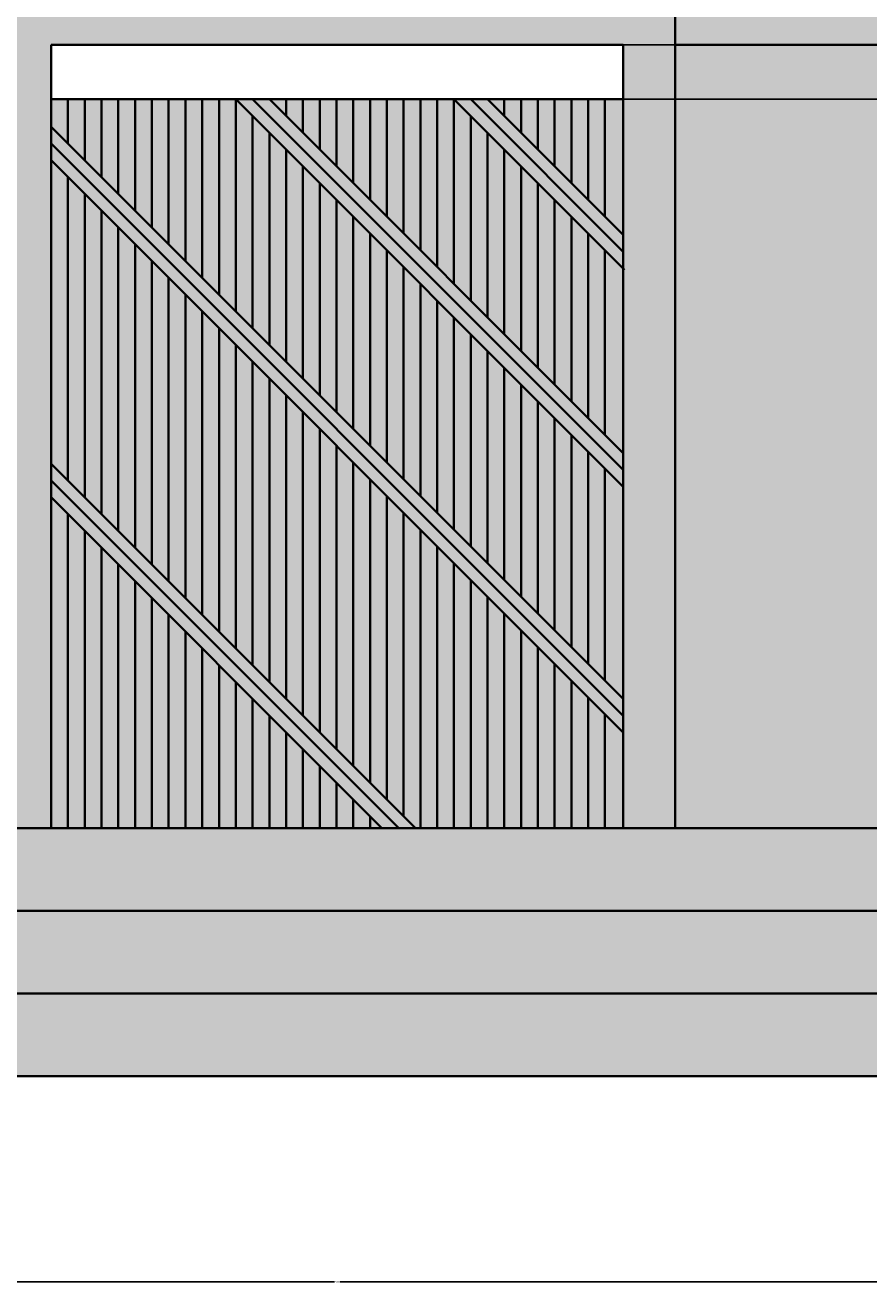
# Model space of a CAD drawing. Units: feet. Extents: x 2893 to 4112, y 897 to 1573.
# Tile 2 of 7: x 3123 to 3253, y 897 to 1090. Entities that reach past the tile are written whole.
import ezdxf

# ---------------------------------------------------------------- set-up
doc = ezdxf.new("R2010")
doc.units = ezdxf.units.FT
for name, color, linetype, lineweight in [('A-ANNO-DIMS', 2, 'Continuous', 18), ('A-ELEV', 7, 'Continuous', 35), ('A-ELEV-PATT', 8, 'Continuous', 13)]:
    doc.layers.add(name, color=color, linetype=linetype, lineweight=lineweight)
doc.styles.get("Standard").update_dxf_attribs({"font": 'arial.ttf'})
doc.dimstyles.get("Standard").update_dxf_attribs({"dimtxt": 0.18, "dimasz": 0.18, "dimexe": 0.18, "dimexo": 0.0625, "dimgap": 0.09, "dimtad": 0, "dimtih": 1, "dimtoh": 1, "dimdec": 1, "dimzin": 0, "dimdsep": 46, "dimlunit": 3, "dimtxsty": 'Standard', "dimcen": 0.09, "dimadec": 0, "dimazin": 0, "dimtfac": 1, "dimtdec": 1, "dimtofl": 0, "dimtmove": 0, "dimatfit": 3, "dimfxl": 1, "dimtolj": 1, "dimtzin": 0, "dimarcsym": 0})

# ---------------------------------------------------------------- blocks, each defined once
blk = doc.blocks.new('*D48')
at = {"layer": 'A-ANNO-DIMS', "color": 0, "lineweight": -2, "transparency": 16777216}
for p, q in [((2924.72, 1491.83), (2924.72, 897.37)), ((3417.56, 1491.83), (3417.56, 897.37)), ((2924.9, 897.55), (3170.74, 897.55)), ((3417.38, 897.55), (3171.54, 897.55))]:
    blk.add_line(p, q, dxfattribs=at)
at = {"layer": 'A-ANNO-DIMS', "color": 0, "transparency": 16777216}
for points in [[(2924.9, 897.58), (2924.9, 897.52), (2924.72, 897.55)], [(3417.38, 897.58), (3417.38, 897.52), (3417.56, 897.55)]]:
    blk.add_solid(points, dxfattribs=at)
at = {"layer": 'Defpoints', "color": 0, "transparency": 16777216}
for p in [(2924.72, 1491.89), (3417.56, 1491.89), (3417.56, 897.55)]:
    blk.add_point(p, dxfattribs=at)
at = {"layer": 'A-ANNO-DIMS', "color": 0, "transparency": 16777216, "insert": (3171.14, 897.55), "char_height": 0.18, "attachment_point": 5}
blk.add_mtext('\\A1;492.8', dxfattribs=at)
blk = doc.blocks.new('*D49')
at = {"layer": 'A-ANNO-DIMS', "color": 0, "lineweight": -2, "transparency": 16777216}
for p, q in [((3215.03, 1078.68), (3449.24, 1078.68)), ((3449.06, 1078.5), (3449.06, 1023.03)), ((3449.06, 967.19), (3449.06, 1022.66)), ((3215.03, 967.01), (3449.24, 967.01))]:
    blk.add_line(p, q, dxfattribs=at)
at = {"layer": 'A-ANNO-DIMS', "color": 0, "transparency": 16777216}
for points in [[(3449.03, 1078.5), (3449.09, 1078.5), (3449.06, 1078.68)], [(3449.03, 967.19), (3449.09, 967.19), (3449.06, 967.01)]]:
    blk.add_solid(points, dxfattribs=at)
at = {"layer": 'Defpoints', "color": 0, "transparency": 16777216}
for p in [(3214.97, 1078.68), (3449.06, 1078.68), (3214.97, 967.01)]:
    blk.add_point(p, dxfattribs=at)
at = {"layer": 'A-ANNO-DIMS', "color": 0, "transparency": 16777216, "insert": (3449.06, 1022.85), "char_height": 0.18, "attachment_point": 5}
blk.add_mtext('\\A1;111.66', dxfattribs=at)
blk = doc.blocks.new('*D50')
at = {"layer": 'A-ANNO-DIMS', "color": 0, "lineweight": -2, "transparency": 16777216}
for p, q in [((3215.03, 1087.01), (3449.24, 1087.01)), ((3449.06, 1086.83), (3449.06, 1083.03)), ((3449.06, 1078.86), (3449.06, 1082.66)), ((3215.03, 1078.68), (3449.24, 1078.68))]:
    blk.add_line(p, q, dxfattribs=at)
at = {"layer": 'A-ANNO-DIMS', "color": 0, "transparency": 16777216}
for points in [[(3449.03, 1086.83), (3449.09, 1086.83), (3449.06, 1087.01)], [(3449.03, 1078.86), (3449.09, 1078.86), (3449.06, 1078.68)]]:
    blk.add_solid(points, dxfattribs=at)
at = {"layer": 'Defpoints', "color": 0, "transparency": 16777216}
for p in [(3214.97, 1087.01), (3449.06, 1087.01), (3214.97, 1078.68)]:
    blk.add_point(p, dxfattribs=at)
at = {"layer": 'A-ANNO-DIMS', "color": 0, "transparency": 16777216, "insert": (3449.06, 1082.85), "char_height": 0.18, "attachment_point": 5}
blk.add_mtext('\\A1;8.338', dxfattribs=at)
blk = doc.blocks.new('*D51')
at = {"layer": 'A-ANNO-DIMS', "color": 0, "lineweight": -2, "transparency": 16777216}
for p, q in [((3189.38, 1112.11), (3449.24, 1112.11)), ((3449.06, 1111.93), (3449.06, 1099.74)), ((3449.06, 1087.19), (3449.06, 1099.38)), ((3215.03, 1087.01), (3449.24, 1087.01))]:
    blk.add_line(p, q, dxfattribs=at)
at = {"layer": 'A-ANNO-DIMS', "color": 0, "transparency": 16777216}
for points in [[(3449.03, 1111.93), (3449.09, 1111.93), (3449.06, 1112.11)], [(3449.03, 1087.19), (3449.09, 1087.19), (3449.06, 1087.01)]]:
    blk.add_solid(points, dxfattribs=at)
at = {"layer": 'Defpoints', "color": 0, "transparency": 16777216}
for p in [(3189.32, 1112.11), (3449.06, 1112.11), (3214.97, 1087.01)]:
    blk.add_point(p, dxfattribs=at)
at = {"layer": 'A-ANNO-DIMS', "color": 0, "transparency": 16777216, "insert": (3449.06, 1099.56), "char_height": 0.18, "attachment_point": 5}
blk.add_mtext('\\A1;25.095', dxfattribs=at)

msp = doc.modelspace()

# ---------------------------------------------------------------- hatches: boundary and pattern name
at = {"layer": 'A-ELEV-PATT'}
h = msp.add_hatch(color=256, dxfattribs=at)
h.dxf.hatch_style = 1
h.paths.add_polyline_path([(3222.9589, 1541.1646), (3119.3255, 1541.1646), (3119.3255, 967.0143), (3127.3151, 967.0143), (3127.3151, 1087.0143), (3214.9693, 1087.0143), (3214.9693, 1078.6766), (3214.9693, 967.0143), (3222.9589, 967.0143)])
h.paths.add_polyline_path([(3152.9675, 1482.3616), (3189.3169, 1482.3616), (3189.3169, 1457.0324), (3189.3169, 1377.2236), (3152.9675, 1377.2236), (3152.9675, 1457.0324)], flags=16)
h.paths.add_polyline_path([(3155.237, 1480.0922), (3187.0474, 1480.0922), (3187.0474, 1459.3019), (3155.237, 1459.3019)], flags=0)
h.paths.add_polyline_path([(3155.237, 1454.7629), (3187.0474, 1454.7629), (3187.0474, 1379.4931), (3155.237, 1379.4931)], flags=0)
h.paths.add_polyline_path([(3152.9675, 1354.8437), (3189.3169, 1354.8437), (3189.3169, 1329.5145), (3189.3169, 1249.7057), (3152.9675, 1249.7057), (3152.9675, 1329.5145)], flags=16)
h.paths.add_polyline_path([(3155.237, 1352.5742), (3187.0474, 1352.5742), (3187.0474, 1331.784), (3155.237, 1331.784)], flags=0)
h.paths.add_polyline_path([(3155.237, 1327.245), (3187.0474, 1327.245), (3187.0474, 1251.9752), (3155.237, 1251.9752)], flags=0)
h.paths.add_polyline_path([(3152.9675, 1217.2478), (3189.3169, 1217.2478), (3189.3169, 1191.9186), (3189.3169, 1112.1098), (3152.9675, 1112.1098), (3152.9675, 1191.9186)], flags=16)
h.paths.add_polyline_path([(3155.237, 1214.9783), (3187.0474, 1214.9783), (3187.0474, 1194.1881), (3155.237, 1194.1881)], flags=0)
h.paths.add_polyline_path([(3155.237, 1189.6491), (3187.0474, 1189.6491), (3187.0474, 1114.3793), (3155.237, 1114.3793)], flags=0)
h = msp.add_hatch(dxfattribs=at)
h.set_pattern_fill('AR-BRELM', color=256, scale=0.1)
h.set_pattern_definition([(0, (-663.002, 0), (0, 13.5484), [19.3675, -0.9525]), (0, (-663.002, 5.715), (0, 13.5484), [19.3675, -0.9525]), (0, (-657.922, 6.774), (0, 13.5484), [9.2075, -0.9525]), (0, (-657.922, 12.489), (0, 13.5484), [9.2075, -0.9525]), (90, (-663.002, 0), (-20.32, 1e-15), [5.715, -7.8334]), (90, (-663.954, 0), (-20.32, 1e-15), [5.715, -7.8334]), (90, (-657.922, 6.774), (-10.16, 6e-16), [5.715, -7.8334]), (90, (-658.874, 6.774), (-10.16, 6e-16), [5.715, -7.8334])])
h.paths.add_polyline_path([(3222.9589, 1541.1646), (3119.3255, 1541.1646), (3119.3255, 967.0143), (3127.3151, 967.0143), (3127.3151, 1087.0143), (3214.9693, 1087.0143), (3214.9693, 1078.6766), (3214.9693, 967.0143), (3222.9589, 967.0143)])
h.paths.add_polyline_path([(3152.9675, 1482.3616), (3189.3169, 1482.3616), (3189.3169, 1457.0324), (3189.3169, 1377.2236), (3152.9675, 1377.2236), (3152.9675, 1457.0324)], flags=16)
h.paths.add_polyline_path([(3155.237, 1480.0922), (3187.0474, 1480.0922), (3187.0474, 1459.3019), (3155.237, 1459.3019)], flags=0)
h.paths.add_polyline_path([(3155.237, 1454.7629), (3187.0474, 1454.7629), (3187.0474, 1379.4931), (3155.237, 1379.4931)], flags=0)
h.paths.add_polyline_path([(3152.9675, 1354.8437), (3189.3169, 1354.8437), (3189.3169, 1329.5145), (3189.3169, 1249.7057), (3152.9675, 1249.7057), (3152.9675, 1329.5145)], flags=16)
h.paths.add_polyline_path([(3155.237, 1352.5742), (3187.0474, 1352.5742), (3187.0474, 1331.784), (3155.237, 1331.784)], flags=0)
h.paths.add_polyline_path([(3155.237, 1327.245), (3187.0474, 1327.245), (3187.0474, 1251.9752), (3155.237, 1251.9752)], flags=0)
h.paths.add_polyline_path([(3152.9675, 1217.2478), (3189.3169, 1217.2478), (3189.3169, 1191.9186), (3189.3169, 1112.1098), (3152.9675, 1112.1098), (3152.9675, 1191.9186)], flags=16)
h.paths.add_polyline_path([(3155.237, 1214.9783), (3187.0474, 1214.9783), (3187.0474, 1194.1881), (3155.237, 1194.1881)], flags=0)
h.paths.add_polyline_path([(3155.237, 1189.6491), (3187.0474, 1189.6491), (3187.0474, 1114.3793), (3155.237, 1114.3793)], flags=0)
h = msp.add_hatch(color=256, dxfattribs=at)
h.dxf.hatch_style = 1
h.paths.add_polyline_path([(3119.3255, 1527.889), (2924.7207, 1527.889), (2924.7207, 1491.889), (3119.3255, 1491.889)])
h.paths.add_polyline_path([(3417.5637, 1527.889), (3222.9589, 1527.889), (3222.9589, 1491.889), (3417.5637, 1491.889)])
h.paths.add_polyline_path([(3119.3255, 1102.9302), (2946.0771, 1102.9302), (2946.0771, 1139.3799), (2934.0287, 1139.3799), (2934.0287, 1093.0143), (3119.3255, 1093.0143)])
h.paths.add_polyline_path([(3119.3255, 1093.0143), (2934.4679, 1093.0143), (2934.4679, 1087.0143), (3119.3255, 1087.0143)])
h.paths.add_polyline_path([(3408.2557, 1139.3799), (3396.2073, 1139.3799), (3396.2073, 1136.9984), (3396.2073, 1102.9302), (3222.9589, 1102.9302), (3222.9589, 1093.0143), (3408.2557, 1093.0143)])
h.paths.add_polyline_path([(3407.8165, 1093.0143), (3222.9589, 1093.0143), (3222.9589, 1087.0143), (3407.8165, 1087.0143)])
h = msp.add_hatch(color=256, dxfattribs=at)
h.dxf.hatch_style = 1
h.paths.add_polyline_path([(3390.4511, 1087.0143), (3222.9589, 1087.0143), (3222.9589, 967.0143), (3255.8959, 967.0143), (3255.8959, 1053.0375), (3262.7641, 1053.0375), (3364.4735, 1053.0375), (3364.4735, 967.0143), (3390.4511, 967.0143)])
h.paths.add_polyline_path([(3119.3255, 1087.0143), (2951.8333, 1087.0143), (2951.8333, 967.0143), (2977.8109, 967.0143), (2977.8109, 1053.0375), (2984.6791, 1053.0375), (3086.3885, 1053.0375), (3086.3885, 967.0143), (3119.3255, 967.0143)])
h = msp.add_hatch(color=256, dxfattribs=at)
h.dxf.hatch_style = 1
h.paths.add_polyline_path([(3189.0392, 1078.6766), (3186.4674, 1078.6766), (3186.4674, 1052.9582), (3189.0392, 1050.3864)], flags=16)
h.paths.add_polyline_path([(3186.4674, 1078.6766), (3183.8955, 1078.6766), (3183.8955, 1055.5301), (3186.4674, 1052.9582)], flags=16)
h.paths.add_polyline_path([(3183.8955, 1078.6766), (3181.3237, 1078.6766), (3181.3237, 1058.1019), (3183.8955, 1055.5301)], flags=16)
h.paths.add_polyline_path([(3181.3237, 1078.6766), (3178.7518, 1078.6766), (3178.7518, 1060.6737), (3181.3237, 1058.1019)], flags=16)
h.paths.add_polyline_path([(3178.7518, 1078.6766), (3176.18, 1078.6766), (3176.18, 1063.2456), (3178.7518, 1060.6737)], flags=16)
h.paths.add_polyline_path([(3176.18, 1078.6766), (3173.6082, 1078.6766), (3173.6082, 1065.8174), (3176.18, 1063.2456)], flags=16)
h.paths.add_polyline_path([(3173.6082, 1078.6766), (3171.0363, 1078.6766), (3171.0363, 1068.3892), (3173.6082, 1065.8174)], flags=16)
h.paths.add_polyline_path([(3171.0363, 1078.6766), (3168.4645, 1078.6766), (3168.4645, 1070.9611), (3171.0363, 1068.3892)], flags=16)
h.paths.add_polyline_path([(3168.4645, 1078.6766), (3165.8926, 1078.6766), (3165.8926, 1073.5329), (3168.4645, 1070.9611)], flags=16)
h.paths.add_polyline_path([(3165.8926, 1078.6766), (3163.3208, 1078.6766), (3163.3208, 1076.1048), (3165.8926, 1073.5329)], flags=16)
h.paths.add_polyline_path([(3163.3208, 1078.6766), (3160.749, 1078.6766), (3163.3208, 1076.1048)], flags=16)
h.paths.add_polyline_path([(3160.749, 1078.6766), (3158.1771, 1078.6766), (3214.9693, 1021.8844), (3214.9693, 1024.4562)], flags=17)
h.paths.add_polyline_path([(3158.1771, 1078.6766), (3155.6053, 1078.6766), (3214.9693, 1019.3125), (3214.9693, 1021.8844)])
h.paths.add_polyline_path([(3196.7547, 1037.5272), (3194.1829, 1040.099), (3194.1829, 1007.596), (3196.7547, 1005.0242)], flags=17)
h.paths.add_polyline_path([(3199.3266, 1034.9553), (3196.7547, 1037.5272), (3196.7547, 1005.0242), (3199.3266, 1002.4523)], flags=17)
h.paths.add_polyline_path([(3201.8984, 1032.3835), (3199.3266, 1034.9553), (3199.3266, 1002.4523), (3201.8984, 999.8805)], flags=17)
h.paths.add_polyline_path([(3204.4702, 1029.8117), (3201.8984, 1032.3835), (3201.8984, 999.8805), (3204.4702, 997.3086)], flags=17)
h.paths.add_polyline_path([(3207.0421, 1027.2398), (3204.4702, 1029.8117), (3204.4702, 997.3086), (3207.0421, 994.7368)], flags=17)
h.paths.add_polyline_path([(3209.6139, 1024.668), (3207.0421, 1027.2398), (3207.0421, 994.7368), (3209.6139, 992.165)], flags=17)
h.paths.add_polyline_path([(3212.1857, 1022.0961), (3209.6139, 1024.668), (3209.6139, 992.165), (3212.1857, 989.5931)], flags=17)
h.paths.add_polyline_path([(3214.9693, 1019.3125), (3212.1857, 1022.0961), (3212.1857, 989.5931), (3214.9693, 986.8095)], flags=17)
h.paths.add_polyline_path([(3173.6082, 1060.6737), (3171.0363, 1063.2456), (3171.0363, 1030.7426), (3173.6082, 1028.1707)], flags=17)
h.paths.add_polyline_path([(3176.18, 1058.1019), (3173.6082, 1060.6737), (3173.6082, 1028.1707), (3176.18, 1025.5989)], flags=17)
h.paths.add_polyline_path([(3178.7518, 1055.5301), (3176.18, 1058.1019), (3176.18, 1025.5989), (3178.7518, 1023.027)], flags=17)
h.paths.add_polyline_path([(3181.3237, 1052.9582), (3178.7518, 1055.5301), (3178.7518, 1023.027), (3181.3237, 1020.4552)], flags=17)
h.paths.add_polyline_path([(3183.8955, 1050.3864), (3181.3237, 1052.9582), (3181.3237, 1020.4552), (3183.8955, 1017.8834)], flags=17)
h.paths.add_polyline_path([(3186.4674, 1047.8145), (3183.8955, 1050.3864), (3183.8955, 1017.8834), (3186.4674, 1015.3115)], flags=17)
h.paths.add_polyline_path([(3189.0392, 1045.2427), (3186.4674, 1047.8145), (3186.4674, 1015.3115), (3189.0392, 1012.7397)], flags=17)
h.paths.add_polyline_path([(3191.611, 1042.6709), (3189.0392, 1045.2427), (3189.0392, 1012.7397), (3191.611, 1010.1678)], flags=17)
h.paths.add_polyline_path([(3194.1829, 1040.099), (3191.611, 1042.6709), (3191.611, 1010.1678), (3194.1829, 1007.596)], flags=17)
h.paths.add_polyline_path([(3171.0363, 1063.2456), (3168.4645, 1065.8174), (3168.4645, 1033.3144), (3171.0363, 1030.7426)], flags=17)
h.paths.add_polyline_path([(3168.4645, 1065.8174), (3165.8926, 1068.3892), (3165.8926, 1035.8862), (3168.4645, 1033.3144)], flags=17)
h.paths.add_polyline_path([(3165.8926, 1068.3892), (3163.3208, 1070.9611), (3163.3208, 1038.4581), (3165.8926, 1035.8862)], flags=17)
h.paths.add_polyline_path([(3163.3208, 1070.9611), (3160.749, 1073.5329), (3160.749, 1041.0299), (3163.3208, 1038.4581)], flags=17)
h.paths.add_polyline_path([(3160.749, 1073.5329), (3158.1771, 1076.1048), (3158.1771, 1043.6018), (3160.749, 1041.0299)], flags=16)
h.paths.add_polyline_path([(3158.1771, 1076.1048), (3155.6053, 1078.6766), (3155.6053, 1046.1736), (3158.1771, 1043.6018)], flags=17)
h.paths.add_polyline_path([(3155.6053, 1078.6766), (3153.0334, 1078.6766), (3153.0334, 1048.7454), (3155.6053, 1046.1736)])
h.paths.add_polyline_path([(3153.0334, 1078.6766), (3150.4616, 1078.6766), (3150.4616, 1051.3173), (3153.0334, 1048.7454)])
h.paths.add_polyline_path([(3150.4616, 1078.6766), (3147.8898, 1078.6766), (3147.8898, 1053.8891), (3150.4616, 1051.3173)])
h.paths.add_polyline_path([(3147.8898, 1078.6766), (3145.3179, 1078.6766), (3145.3179, 1056.4609), (3147.8898, 1053.8891)])
h.paths.add_polyline_path([(3145.3179, 1078.6766), (3142.7461, 1078.6766), (3142.7461, 1059.0328), (3145.3179, 1056.4609)])
h.paths.add_polyline_path([(3140.1742, 1078.6766), (3137.6024, 1078.6766), (3137.6024, 1064.1765), (3140.1742, 1061.6046)])
h.paths.add_polyline_path([(3142.7461, 1078.6766), (3140.1742, 1078.6766), (3140.1742, 1061.6046), (3142.7461, 1059.0328)])
h.paths.add_polyline_path([(3137.6024, 1078.6766), (3135.0306, 1078.6766), (3135.0306, 1066.7483), (3137.6024, 1064.1765)])
h.paths.add_polyline_path([(3135.0306, 1078.6766), (3132.4587, 1078.6766), (3132.4587, 1069.3201), (3135.0306, 1066.7483)])
h.paths.add_polyline_path([(3129.8869, 1078.6766), (3127.3151, 1078.6766), (3127.3151, 1074.4638), (3129.8869, 1071.892)])
h.paths.add_polyline_path([(3132.4587, 1078.6766), (3129.8869, 1078.6766), (3129.8869, 1071.892), (3132.4587, 1069.3201)])
h.paths.add_polyline_path([(3127.3151, 1074.4638), (3127.3151, 1071.892), (3214.9693, 984.2377), (3214.9693, 986.8095)])
h.paths.add_polyline_path([(3176.18, 968.8368), (3176.18, 967.0143), (3178.0025, 967.0143)], flags=16)
h.paths.add_polyline_path([(3176.18, 968.8368), (3173.6082, 971.4087), (3173.6082, 967.0143), (3176.18, 967.0143)], flags=16)
h.paths.add_polyline_path([(3173.6082, 971.4087), (3171.0363, 973.9805), (3171.0363, 967.0143), (3173.6082, 967.0143)], flags=16)
h.paths.add_polyline_path([(3171.0363, 973.9805), (3168.4645, 976.5524), (3168.4645, 967.0143), (3171.0363, 967.0143)], flags=16)
h.paths.add_polyline_path([(3168.4645, 976.5524), (3165.8926, 979.1242), (3165.8926, 967.0143), (3168.4645, 967.0143)], flags=16)
h.paths.add_polyline_path([(3165.8926, 979.1242), (3163.3208, 981.696), (3163.3208, 967.0143), (3165.8926, 967.0143)], flags=16)
h.paths.add_polyline_path([(3163.3208, 981.696), (3160.749, 984.2679), (3160.749, 967.0143), (3163.3208, 967.0143)], flags=16)
h.paths.add_polyline_path([(3160.749, 984.2679), (3158.1771, 986.8397), (3158.1771, 967.0143), (3160.749, 967.0143)], flags=16)
h.paths.add_polyline_path([(3158.1771, 986.8397), (3155.6053, 989.4116), (3155.6053, 967.0143), (3158.1771, 967.0143)], flags=16)
h.paths.add_polyline_path([(3155.6053, 989.4116), (3153.0334, 991.9834), (3153.0334, 967.0143), (3155.6053, 967.0143)], flags=16)
h.paths.add_polyline_path([(3153.0334, 991.9834), (3150.4616, 994.5552), (3150.4616, 967.0143), (3153.0334, 967.0143)], flags=16)
h.paths.add_polyline_path([(3127.3151, 1020.2736), (3127.3151, 1017.7018), (3178.0025, 967.0143), (3180.5744, 967.0143)], flags=17)
h.paths.add_polyline_path([(3127.3151, 1022.8455), (3127.3151, 1020.2736), (3180.5744, 967.0143), (3183.1462, 967.0143)])
h = msp.add_hatch(color=256, dxfattribs=at)
h.dxf.hatch_style = 1
h.paths.add_polyline_path([(3214.9693, 1078.6766), (3212.1857, 1078.6766), (3212.1857, 1060.6737), (3214.9693, 1057.8901)], flags=16)
h.paths.add_polyline_path([(3212.1857, 1078.6766), (3209.6139, 1078.6766), (3209.6139, 1063.2456), (3212.1857, 1060.6737)], flags=16)
h.paths.add_polyline_path([(3209.6139, 1078.6766), (3207.0421, 1078.6766), (3207.0421, 1065.8174), (3209.6139, 1063.2456)], flags=16)
h.paths.add_polyline_path([(3207.0421, 1078.6766), (3204.4702, 1078.6766), (3204.4702, 1068.3892), (3207.0421, 1065.8174)], flags=16)
h.paths.add_polyline_path([(3204.4702, 1078.6766), (3201.8984, 1078.6766), (3201.8984, 1070.9611), (3204.4702, 1068.3892)], flags=16)
h.paths.add_polyline_path([(3201.8984, 1078.6766), (3199.3266, 1078.6766), (3199.3266, 1073.5329), (3201.8984, 1070.9611)], flags=16)
h.paths.add_polyline_path([(3199.3266, 1078.6766), (3196.7547, 1078.6766), (3196.7547, 1076.1048), (3199.3266, 1073.5329)], flags=16)
h.paths.add_polyline_path([(3196.7547, 1078.6766), (3194.1829, 1078.6766), (3196.7547, 1076.1048)], flags=16)
h.paths.add_polyline_path([(3196.7547, 1076.1048), (3194.1829, 1078.6766), (3191.611, 1078.6766), (3214.9693, 1055.3183), (3214.9693, 1057.8901), (3212.1857, 1060.6737), (3209.6139, 1063.2456), (3207.0421, 1065.8174), (3204.4702, 1068.3892), (3201.8984, 1070.9611), (3199.3266, 1073.5329)], flags=17)
h.paths.add_polyline_path([(3191.611, 1078.6766), (3189.0392, 1078.6766), (3214.9693, 1052.7465), (3214.9693, 1055.3183)])
h.paths.add_polyline_path([(3214.9693, 1052.7465), (3212.1857, 1055.5301), (3212.1857, 1027.2398), (3214.9693, 1024.4562)])
h.paths.add_polyline_path([(3212.1857, 1055.5301), (3209.6139, 1058.1019), (3209.6139, 1029.8117), (3212.1857, 1027.2398)])
h.paths.add_polyline_path([(3209.6139, 1058.1019), (3207.0421, 1060.6737), (3207.0421, 1032.3835), (3209.6139, 1029.8117)])
h.paths.add_polyline_path([(3207.0421, 1060.6737), (3204.4702, 1063.2456), (3204.4702, 1034.9553), (3207.0421, 1032.3835)])
h.paths.add_polyline_path([(3204.4702, 1063.2456), (3201.8984, 1065.8174), (3201.8984, 1037.5272), (3204.4702, 1034.9553)])
h.paths.add_polyline_path([(3201.8984, 1065.8174), (3199.3266, 1068.3892), (3199.3266, 1040.099), (3201.8984, 1037.5272)])
h.paths.add_polyline_path([(3199.3266, 1068.3892), (3196.7547, 1070.9611), (3196.7547, 1042.6709), (3199.3266, 1040.099)])
h.paths.add_polyline_path([(3196.7547, 1070.9611), (3194.1829, 1073.5329), (3194.1829, 1045.2427), (3196.7547, 1042.6709)])
h.paths.add_polyline_path([(3194.1829, 1073.5329), (3191.611, 1076.1048), (3191.611, 1047.8145), (3194.1829, 1045.2427)])
h.paths.add_polyline_path([(3191.611, 1076.1048), (3189.0392, 1078.6766), (3189.0392, 1050.3864), (3191.611, 1047.8145)])
h = msp.add_hatch(color=256, dxfattribs=at)
h.dxf.hatch_style = 1
h.paths.add_polyline_path([(3129.8869, 1015.13), (3127.3151, 1017.7018), (3127.3151, 967.0143), (3129.8869, 967.0143)])
h.paths.add_polyline_path([(3132.4587, 1012.5581), (3129.8869, 1015.13), (3129.8869, 967.0143), (3132.4587, 967.0143)])
h.paths.add_polyline_path([(3135.0306, 1009.9863), (3132.4587, 1012.5581), (3132.4587, 967.0143), (3135.0306, 967.0143)])
h.paths.add_polyline_path([(3137.6024, 1007.4144), (3135.0306, 1009.9863), (3135.0306, 967.0143), (3137.6024, 967.0143)])
h.paths.add_polyline_path([(3173.6082, 1023.027), (3171.0363, 1025.5989), (3171.0363, 979.1242), (3173.6082, 976.5524)])
h.paths.add_polyline_path([(3171.0363, 1025.5989), (3168.4645, 1028.1707), (3168.4645, 981.696), (3171.0363, 979.1242)])
h.paths.add_polyline_path([(3168.4645, 1028.1707), (3165.8926, 1030.7426), (3165.8926, 984.2679), (3168.4645, 981.696)], flags=17)
h.paths.add_polyline_path([(3165.8926, 1030.7426), (3163.3208, 1033.3144), (3163.3208, 986.8397), (3165.8926, 984.2679)], flags=17)
h.paths.add_polyline_path([(3163.3208, 1033.3144), (3160.749, 1035.8862), (3160.749, 989.4116), (3163.3208, 986.8397)], flags=17)
h.paths.add_polyline_path([(3160.749, 1035.8862), (3158.1771, 1038.4581), (3158.1771, 991.9834), (3160.749, 989.4116)], flags=17)
h.paths.add_polyline_path([(3158.1771, 1038.4581), (3155.6053, 1041.0299), (3155.6053, 994.5552), (3158.1771, 991.9834)], flags=17)
h.paths.add_polyline_path([(3155.6053, 1041.0299), (3153.0334, 1043.6018), (3153.0334, 997.1271), (3155.6053, 994.5552)], flags=17)
h.paths.add_polyline_path([(3153.0334, 1043.6018), (3150.4616, 1046.1736), (3150.4616, 999.6989), (3153.0334, 997.1271)], flags=17)
h.paths.add_polyline_path([(3150.4616, 1046.1736), (3147.8898, 1048.7454), (3147.8898, 1002.2708), (3150.4616, 999.6989)], flags=17)
h.paths.add_polyline_path([(3147.8898, 1048.7454), (3145.3179, 1051.3173), (3145.3179, 1004.8426), (3147.8898, 1002.2708)], flags=17)
h.paths.add_polyline_path([(3145.3179, 1051.3173), (3142.7461, 1053.8891), (3142.7461, 1007.4144), (3145.3179, 1004.8426)], flags=17)
h.paths.add_polyline_path([(3142.7461, 1053.8891), (3140.1742, 1056.4609), (3140.1742, 1009.9863), (3142.7461, 1007.4144)], flags=17)
h.paths.add_polyline_path([(3140.1742, 1056.4609), (3137.6024, 1059.0328), (3137.6024, 1012.5581), (3140.1742, 1009.9863)], flags=17)
h.paths.add_polyline_path([(3137.6024, 1059.0328), (3135.0306, 1061.6046), (3135.0306, 1015.13), (3137.6024, 1012.5581)], flags=17)
h.paths.add_polyline_path([(3127.3151, 1071.892), (3127.3151, 1069.3201), (3214.9693, 981.6659), (3214.9693, 984.2377)])
h = msp.add_hatch(color=256, dxfattribs=at)
h.dxf.hatch_style = 1
h.paths.add_polyline_path([(3132.4587, 1064.1765), (3129.8869, 1066.7483), (3129.8869, 1020.2736), (3132.4587, 1017.7018)])
h.paths.add_polyline_path([(3135.0306, 1061.6046), (3132.4587, 1064.1765), (3132.4587, 1017.7018), (3135.0306, 1015.13)])
h.paths.add_polyline_path([(3129.8869, 1066.7483), (3127.3151, 1069.3201), (3127.3151, 1022.8455), (3129.8869, 1020.2736)])
h = msp.add_hatch(color=256, dxfattribs=at)
h.dxf.hatch_style = 1
h.paths.add_polyline_path([(3214.9693, 981.6659), (3212.1857, 984.4494), (3212.1857, 967.0143), (3214.9693, 967.0143)])
h.paths.add_polyline_path([(3212.1857, 984.4494), (3209.6139, 987.0213), (3209.6139, 967.0143), (3212.1857, 967.0143)])
h.paths.add_polyline_path([(3209.6139, 987.0213), (3207.0421, 989.5931), (3207.0421, 967.0143), (3209.6139, 967.0143)])
h.paths.add_polyline_path([(3207.0421, 989.5931), (3204.4702, 992.165), (3204.4702, 967.0143), (3207.0421, 967.0143)])
h.paths.add_polyline_path([(3204.4702, 992.165), (3201.8984, 994.7368), (3201.8984, 967.0143), (3204.4702, 967.0143)])
h.paths.add_polyline_path([(3201.8984, 994.7368), (3199.3266, 997.3086), (3199.3266, 967.0143), (3201.8984, 967.0143)])
h.paths.add_polyline_path([(3199.3266, 997.3086), (3196.7547, 999.8805), (3196.7547, 967.0143), (3199.3266, 967.0143)])
h.paths.add_polyline_path([(3196.7547, 999.8805), (3194.1829, 1002.4523), (3194.1829, 967.0143), (3196.7547, 967.0143)])
h.paths.add_polyline_path([(3194.1829, 1002.4523), (3191.611, 1005.0242), (3191.611, 967.0143), (3194.1829, 967.0143)])
h.paths.add_polyline_path([(3191.611, 1005.0242), (3189.0392, 1007.596), (3189.0392, 967.0143), (3191.611, 967.0143)])
h.paths.add_polyline_path([(3189.0392, 1007.596), (3186.4674, 1010.1678), (3186.4674, 967.0143), (3189.0392, 967.0143)])
h.paths.add_polyline_path([(3186.4674, 1010.1678), (3183.8955, 1012.7397), (3183.8955, 967.0143), (3186.4674, 967.0143)])
h.paths.add_polyline_path([(3183.8955, 1012.7397), (3181.3237, 1015.3115), (3181.3237, 968.8368), (3183.1462, 967.0143), (3183.8955, 967.0143)])
h.paths.add_polyline_path([(3181.3237, 1015.3115), (3178.7518, 1017.8834), (3178.7518, 971.4087), (3181.3237, 968.8368)])
h.paths.add_polyline_path([(3178.7518, 1017.8834), (3176.18, 1020.4552), (3176.18, 973.9805), (3178.7518, 971.4087)])
h.paths.add_polyline_path([(3176.18, 1020.4552), (3173.6082, 1023.027), (3173.6082, 976.5524), (3176.18, 973.9805)])
h.paths.add_polyline_path([(3147.8898, 997.1271), (3145.3179, 999.6989), (3145.3179, 967.0143), (3147.8898, 967.0143)])
h.paths.add_polyline_path([(3150.4616, 994.5552), (3147.8898, 997.1271), (3147.8898, 967.0143), (3150.4616, 967.0143)])
h.paths.add_polyline_path([(3145.3179, 999.6989), (3142.7461, 1002.2708), (3142.7461, 967.0143), (3145.3179, 967.0143)])
h.paths.add_polyline_path([(3142.7461, 1002.2708), (3140.1742, 1004.8426), (3140.1742, 967.0143), (3142.7461, 967.0143)])
h.paths.add_polyline_path([(3140.1742, 1004.8426), (3137.6024, 1007.4144), (3137.6024, 967.0143), (3140.1742, 967.0143)])
h = msp.add_hatch(color=256, dxfattribs=at)
h.dxf.hatch_style = 1
h.paths.add_polyline_path([(3390.4511, 967.0143), (3222.9589, 967.0143), (2951.8333, 967.0143), (2932.7702, 954.3595), (3409.5142, 954.3595)])
h.paths.add_polyline_path([(3409.5142, 954.3595), (2932.7702, 954.3595), (2932.7702, 945.8624), (2926.5072, 941.7047), (3415.7772, 941.7047), (3409.5142, 945.8624)])
h.paths.add_polyline_path([(3415.7772, 941.7047), (2926.5072, 941.7047), (2926.5072, 929.0499), (3415.7772, 929.0499)])

# ---------------------------------------------------------------- linework, layer by layer
at = {"layer": 'A-ELEV'}
for p, q in [((3222.9589, 967.0143), (3222.9589, 1541.1646)), ((3214.9693, 1087.0143), (3127.3151, 1087.0143)), ((3214.9693, 1087.0143), (3127.3151, 1087.0143)), ((3214.9693, 1087.0143), (3127.3151, 1087.0143)), ((3407.8165, 1087.0143), (3222.9589, 1087.0143)), ((3129.8869, 1078.6766), (3129.8869, 1071.892)), ((3132.4587, 1078.6766), (3132.4587, 1069.3201)), ((3135.0306, 1078.6766), (3135.0306, 1066.7483)), ((3137.6024, 1078.6766), (3137.6024, 1064.1765)), ((3140.1742, 1078.6766), (3140.1742, 1061.6046)), ((3142.7461, 1078.6766), (3142.7461, 1059.0328)), ((3145.3179, 1078.6766), (3145.3179, 1056.4609)), ((3147.8898, 1078.6766), (3147.8898, 1053.8891)), ((3150.4616, 1078.6766), (3150.4616, 1051.3173)), ((3153.0334, 1078.6766), (3153.0334, 1048.7454)), ((3158.1771, 1078.6766), (3214.9693, 1021.8844)), ((3160.749, 1078.6766), (3214.9693, 1024.4562)), ((3163.3208, 1078.6766), (3163.3208, 1076.1048)), ((3163.3208, 1078.6766), (3163.3208, 1076.1048)), ((3165.8926, 1078.6766), (3165.8926, 1073.5329)), ((3168.4645, 1078.6766), (3168.4645, 1070.9611)), ((3171.0363, 1078.6766), (3171.0363, 1068.3892)), ((3173.6082, 1078.6766), (3173.6082, 1065.8174)), ((3176.18, 1078.6766), (3176.18, 1063.2456)), ((3178.7518, 1078.6766), (3178.7518, 1060.6737)), ((3181.3237, 1078.6766), (3181.3237, 1058.1019)), ((3183.8955, 1078.6766), (3183.8955, 1055.5301)), ((3186.4674, 1078.6766), (3186.4674, 1052.9582)), ((3191.611, 1078.6766), (3214.9693, 1055.3183)), ((3194.1829, 1078.6766), (3214.9693, 1057.8901)), ((3196.7547, 1078.6766), (3196.7547, 1076.1048)), ((3196.7547, 1078.6766), (3196.7547, 1076.1048)), ((3199.3266, 1078.6766), (3199.3266, 1073.5329)), ((3201.8984, 1078.6766), (3201.8984, 1070.9611)), ((3204.4702, 1078.6766), (3204.4702, 1068.3892)), ((3207.0421, 1078.6766), (3207.0421, 1065.8174)), ((3209.6139, 1078.6766), (3209.6139, 1063.2456)), ((3212.1857, 1078.6766), (3212.1857, 1060.6737)), ((3158.1771, 1076.1048), (3158.1771, 1043.6018)), ((3191.611, 1076.1048), (3191.611, 1047.8145)), ((3127.3151, 1074.4638), (3214.9693, 986.8095)), ((3160.749, 1073.5329), (3160.749, 1041.0299)), ((3194.1829, 1073.5329), (3194.1829, 1045.2427)), ((3127.3151, 1071.892), (3214.9693, 984.2377)), ((3127.3151, 1069.3201), (3214.9693, 981.6659)), ((3163.3208, 1070.9611), (3163.3208, 1038.4581)), ((3196.7547, 1070.9611), (3196.7547, 1042.6709)), ((3165.8926, 1068.3892), (3165.8926, 1035.8862)), ((3199.3266, 1068.3892), (3199.3266, 1040.099)), ((3129.8869, 1066.7483), (3129.8869, 1020.2736)), ((3168.4645, 1065.8174), (3168.4645, 1033.3144)), ((3201.8984, 1065.8174), (3201.8984, 1037.5272)), ((3132.4587, 1064.1765), (3132.4587, 1017.7018)), ((3135.0306, 1061.6046), (3135.0306, 1015.13)), ((3171.0363, 1063.2456), (3171.0363, 1030.7426)), ((3204.4702, 1063.2456), (3204.4702, 1034.9553)), ((3173.6082, 1060.6737), (3173.6082, 1028.1707)), ((3207.0421, 1060.6737), (3207.0421, 1032.3835)), ((3137.6024, 1059.0328), (3137.6024, 1012.5581)), ((3176.18, 1058.1019), (3176.18, 1025.5989)), ((3209.6139, 1058.1019), (3209.6139, 1029.8117)), ((3140.1742, 1056.4609), (3140.1742, 1009.9863)), ((3142.7461, 1053.8891), (3142.7461, 1007.4144)), ((3178.7518, 1055.5301), (3178.7518, 1023.027)), ((3212.1857, 1055.5301), (3212.1857, 1027.2398)), ((3181.3237, 1052.9582), (3181.3237, 1020.4552)), ((3145.3179, 1051.3173), (3145.3179, 1004.8426)), ((3183.8955, 1050.3864), (3183.8955, 1017.8834)), ((3147.8898, 1048.7454), (3147.8898, 1002.2708)), ((3150.4616, 1046.1736), (3150.4616, 999.6989)), ((3186.4674, 1047.8145), (3186.4674, 1015.3115)), ((3189.0392, 1045.2427), (3189.0392, 1012.7397)), ((3153.0334, 1043.6018), (3153.0334, 997.1271)), ((3191.611, 1042.6709), (3191.611, 1010.1678)), ((3155.6053, 1041.0299), (3155.6053, 994.5552)), ((3158.1771, 1038.4581), (3158.1771, 991.9834)), ((3194.1829, 1040.099), (3194.1829, 1007.596)), ((3196.7547, 1037.5272), (3196.7547, 1005.0242)), ((3160.749, 1035.8862), (3160.749, 989.4116)), ((3199.3266, 1034.9553), (3199.3266, 1002.4523)), ((3163.3208, 1033.3144), (3163.3208, 986.8397)), ((3165.8926, 1030.7426), (3165.8926, 984.2679)), ((3201.8984, 1032.3835), (3201.8984, 999.8805)), ((3204.4702, 1029.8117), (3204.4702, 997.3086)), ((3168.4645, 1028.1707), (3168.4645, 981.696)), ((3207.0421, 1027.2398), (3207.0421, 994.7368)), ((3171.0363, 1025.5989), (3171.0363, 979.1242)), ((3173.6082, 1023.027), (3173.6082, 976.5524)), ((3209.6139, 1024.668), (3209.6139, 992.165)), ((3127.3151, 1022.8455), (3183.1462, 967.0143)), ((3212.1857, 1022.0961), (3212.1857, 989.5931)), ((3127.3151, 1020.2736), (3180.5744, 967.0143)), ((3176.18, 1020.4552), (3176.18, 973.9805)), ((3127.3151, 1017.7018), (3178.0025, 967.0143)), ((3178.7518, 1017.8834), (3178.7518, 971.4087)), ((3181.3237, 1015.3115), (3181.3237, 968.8368)), ((3129.8869, 1015.13), (3129.8869, 967.0143)), ((3132.4587, 1012.5581), (3132.4587, 967.0143)), ((3183.8955, 1012.7397), (3183.8955, 967.0143)), ((3135.0306, 1009.9863), (3135.0306, 967.0143)), ((3186.4674, 1010.1678), (3186.4674, 967.0143)), ((3189.0392, 1007.596), (3189.0392, 967.0143)), ((3137.6024, 1007.4144), (3137.6024, 967.0143)), ((3140.1742, 1004.8426), (3140.1742, 967.0143)), ((3191.611, 1005.0242), (3191.611, 967.0143)), ((3142.7461, 1002.2708), (3142.7461, 967.0143)), ((3194.1829, 1002.4523), (3194.1829, 967.0143)), ((3196.7547, 999.8805), (3196.7547, 967.0143)), ((3145.3179, 999.6989), (3145.3179, 967.0143)), ((3147.8898, 997.1271), (3147.8898, 967.0143)), ((3199.3266, 997.3086), (3199.3266, 967.0143)), ((3150.4616, 994.5552), (3150.4616, 967.0143)), ((3201.8984, 994.7368), (3201.8984, 967.0143)), ((3204.4702, 992.165), (3204.4702, 967.0143)), ((3153.0334, 991.9834), (3153.0334, 967.0143)), ((3155.6053, 989.4116), (3155.6053, 967.0143)), ((3207.0421, 989.5931), (3207.0421, 967.0143)), ((3158.1771, 986.8397), (3158.1771, 967.0143)), ((3209.6139, 987.0213), (3209.6139, 967.0143)), ((3212.1857, 984.4494), (3212.1857, 967.0143)), ((3160.749, 984.2679), (3160.749, 967.0143)), ((3163.3208, 981.696), (3163.3208, 967.0143)), ((3165.8926, 979.1242), (3165.8926, 967.0143)), ((3168.4645, 976.5524), (3168.4645, 967.0143)), ((3171.0363, 973.9805), (3171.0363, 967.0143)), ((3173.6082, 971.4087), (3173.6082, 967.0143)), ((3176.18, 968.8368), (3176.18, 967.0143)), ((2951.8333, 967.0143), (3390.4511, 967.0143)), ((2951.8333, 967.0143), (3390.4511, 967.0143))]:
    msp.add_line(p, q, dxfattribs=at)
for points in [[(3119.3255, 967.0143), (3119.3255, 1541.1646), (3222.9589, 1541.1646), (3222.9589, 967.0143)], [(3222.9589, 1093.0143), (3408.2557, 1093.0143), (3408.2557, 1139.3799), (3396.2073, 1139.3799), (3396.2073, 1102.9302), (3222.9589, 1102.9302), (3222.9589, 1087.0143), (3407.8165, 1087.0143), (3407.8165, 1093.0143)], [(3222.9589, 1087.0143), (3222.9589, 1102.9302), (3396.2073, 1102.9302)], [(3155.6053, 1046.1736), (3155.6053, 1078.6766), (3214.9693, 1019.3125)], [(3189.0392, 1050.3864), (3189.0392, 1078.6766), (3215.1785, 1052.5373)], [(2932.7702, 945.8624), (2932.7702, 954.3595), (3409.5142, 954.3595), (3409.5142, 945.8624)], [(2926.5072, 941.7047), (3415.7772, 941.7047)], [(2926.5072, 941.7047), (3415.7772, 941.7047)], [(3409.5142, 941.7047), (2932.7702, 941.7047)], [(3409.5142, 941.7047), (2932.7702, 941.7047)], [(3415.7772, 929.0499), (2926.5072, 929.0499)]]:
    msp.add_lwpolyline(points, dxfattribs=at)
for points in [[(3127.3151, 1087.0143), (3214.9693, 1087.0143), (3214.9693, 967.0143), (3127.3151, 967.0143)], [(3127.3151, 1087.0143), (3214.9693, 1087.0143), (3214.9693, 1078.6766), (3127.3151, 1078.6766)], [(3127.3151, 1087.0143), (3214.9693, 1087.0143), (3214.9693, 967.0143), (3127.3151, 967.0143)], [(3127.3151, 1087.0143), (3214.9693, 1087.0143), (3214.9693, 1078.6766), (3127.3151, 1078.6766)], [(3127.3151, 1087.0143), (3214.9693, 1087.0143), (3214.9693, 967.0143), (3127.3151, 967.0143)], [(3127.3151, 1087.0143), (3214.9693, 1087.0143), (3214.9693, 1078.6766), (3127.3151, 1078.6766)], [(3390.4511, 967.0143), (3222.9589, 967.0143), (3222.9589, 1087.0143), (3390.4511, 1087.0143)], [(3390.4511, 967.0143), (3222.9589, 967.0143), (3222.9589, 1087.0143), (3390.4511, 1087.0143)], [(3127.3151, 1078.6766), (3214.9693, 1078.6766), (3214.9693, 967.0143), (3127.3151, 967.0143)], [(3127.3151, 1078.6766), (3214.9693, 1078.6766), (3214.9693, 967.0143), (3127.3151, 967.0143)], [(2926.5072, 941.7047), (2932.7702, 945.8624), (2932.7702, 954.3595), (3409.5142, 954.3595), (3409.5142, 945.8624), (3415.7772, 941.7047), (3415.7772, 929.0499), (2926.5072, 929.0499)]]:
    msp.add_lwpolyline(points, close=True, dxfattribs=at)

# ---------------------------------------------------------------- dimensions: what is measured, and where the dimension line sits
at = {"layer": 'A-ANNO-DIMS'}
dim = msp.add_linear_dim(base=(3417.5637, 897.5499), p1=(2924.7207, 1491.889), p2=(3417.5637, 1491.889), dimstyle='Standard', override={"dimdec": 1, "dimlfac": 1, "dimrnd": 0, "dimzin": 0, "dimdsep": 46, "dimlunit": 2}, dxfattribs=at)
dim.commit()
dim.dimension.update_dxf_attribs({"geometry": '*D48', "text_midpoint": (3171.1422, 897.5499)})
for base, p1, p2, override, picture, middle in [((3449.06374, 1112.1098), (3214.96934, 1087.01433), (3189.3169, 1112.1098), {"dimdec": 3, "dimlfac": 1, "dimrnd": 0, "dimzin": 0, "dimdsep": 46, "dimlunit": 2}, '*D51', (3449.06374, 1099.56206)), ((3449.0637, 1087.0143), (3214.9693, 1078.6766), (3214.9693, 1087.0143), {"dimdec": 3, "dimlfac": 1, "dimrnd": 0, "dimzin": 0, "dimdsep": 46, "dimlunit": 2}, '*D50', (3449.0637, 1082.8455)), ((3449.0637, 1078.6766), (3214.9693, 967.0143), (3214.9693, 1078.6766), {"dimdec": 2, "dimlfac": 1, "dimrnd": 0, "dimzin": 0, "dimdsep": 46, "dimlunit": 2}, '*D49', (3449.0637, 1022.8455))]:
    dim = msp.add_linear_dim(base=base, p1=p1, p2=p2, angle=90, dimstyle='Standard', override=override, dxfattribs=at)
    dim.commit()
    dim.dimension.update_dxf_attribs({"geometry": picture, "text_midpoint": middle})

doc.saveas('drawing.dxf')
